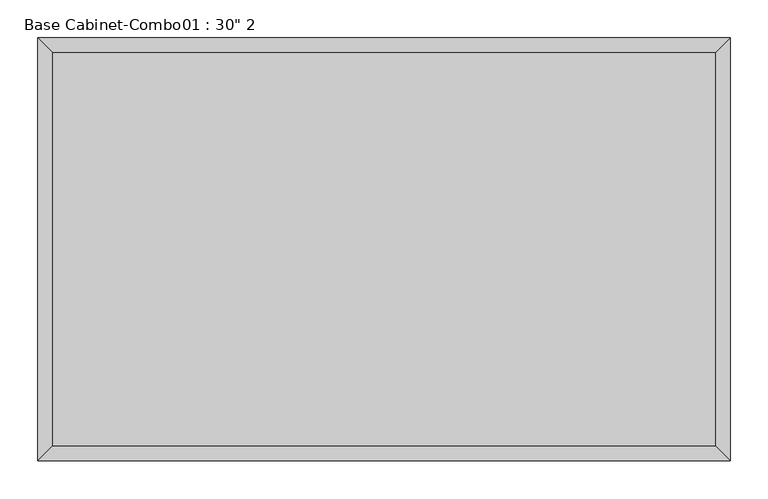
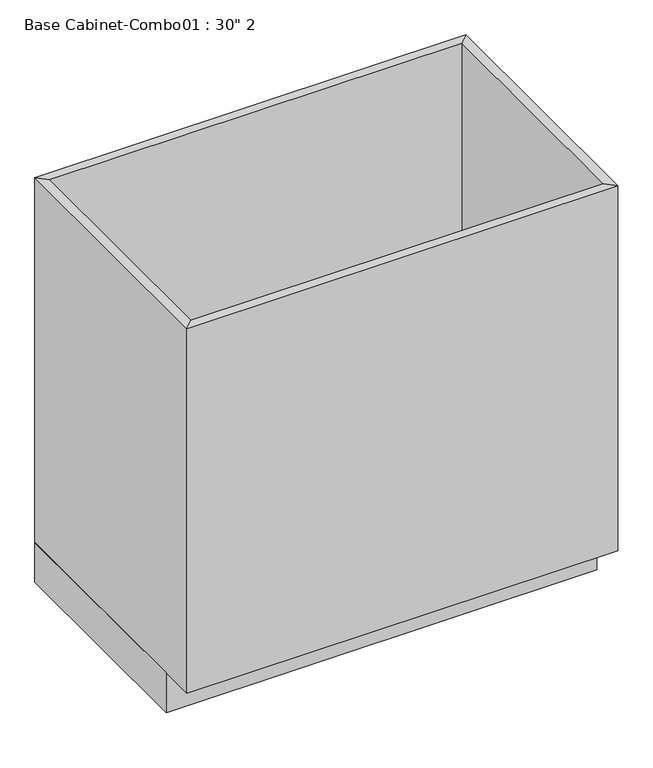
"""IFC4 building model written with IfcOpenShell, lengths in millimetres: furniture geometry."""

from ifc_helpers import new_model, si_unit, frame, origin, origin_with_axes, place, context, project, spatial, polyline, outline, extrude, faceted_brep, source, transform, mapped, element, save


def furniture_f415afdb(model_context):
    return source(origin(), model_context, "Body", "SolidModel", [
        extrude(outline(polyline([(475.9377049, 0.0), (475.9377049, -482.6), (-438.4622951, -482.6), (-438.4622951, 0.0), (475.9377049, 0.0)])), origin_with_axes(), (0.0, 0.0, 1.0), 88.9),
        faceted_brep([(456.8877049, -539.75, 908.05), (456.8877049, -539.75, 88.9), (-419.4122951, -539.75, 88.9), (-419.4122951, -539.75, 908.05), (475.9377049, -558.8, 908.05), (-438.4622951, -558.8, 908.05), (475.9377049, -558.8, 88.9), (-438.4622951, -558.8, 88.9), (-419.4122951, -19.05, 88.9), (-419.4122951, -19.05, 908.05), (-438.4622951, 0.0, 908.05), (-438.4622951, 0.0, 88.9), (456.8877049, -19.05, 88.9), (456.8877049, -19.05, 908.05), (475.9377049, 0.0, 908.05), (475.9377049, 0.0, 88.9)], [[[0, 1, 2, 3]], [[4, 0, 3, 5]], [[6, 4, 5, 7]], [[1, 6, 7, 2]], [[3, 2, 8, 9]], [[5, 3, 9, 10]], [[7, 5, 10, 11]], [[2, 7, 11, 8]], [[9, 8, 12, 13]], [[10, 9, 13, 14]], [[11, 10, 14, 15]], [[8, 11, 15, 12]], [[13, 12, 1, 0]], [[14, 13, 0, 4]], [[15, 14, 4, 6]], [[12, 15, 6, 1]]]),
        extrude(outline(polyline([(456.8877049, -19.05), (456.8877049, -539.75), (-419.4122951, -539.75), (-419.4122951, -19.05), (456.8877049, -19.05)])), frame((0.0, 0.0, 88.9), z_axis=(0.0, 0.0, 1.0), x_axis=(1.0, 0.0, 0.0)), (0.0, 0.0, 1.0), 19.05),
    ])


if __name__ == "__main__":
    model = new_model("IFC4")
    model_context = context("Model", 3, world=origin())
    ifc_project = project(units=[si_unit("LENGTHUNIT", "METRE", prefix="MILLI")], contexts=[model_context])
    site = spatial("IfcSite", under=ifc_project)
    building = spatial("IfcBuilding", under=site)
    placement = place(None, origin())
    furniture_shape = furniture_f415afdb(model_context)
    element("IfcFurniture", 1, ObjectType="Base Cabinet-Combo01 : 30\" 2", at=placement, inside=building, context=model_context, shape_type="MappedRepresentation", body=[
        mapped(furniture_shape, transform((0.0, 0.0, 0.0), x_axis=(1.0, 0.0, 0.0), y_axis=(0.0, 1.0, 0.0), z_axis=(0.0, 0.0, 1.0))),
    ])
    save(model, "model.ifc")

# Revit data of these elements
# Type "Base Cabinet-Combo01 : 30\" 2"
#   Depth = 1' - 10"
#   Height = 2' - 11 3/4"
#   Toe Depth = 0' - 3"
#   Toe Height = 0' - 3 1/2"
#   Width = 3' - 0"
#   Default Elevation = 0
# Element 1 (IfcFurniture, "Base Cabinet-Combo01 : 30\" 2")
#   Materials on its faces: "Cabinet"
# Materials
#   "Cabinet": colour RGB 204 122 2, transparency 0
